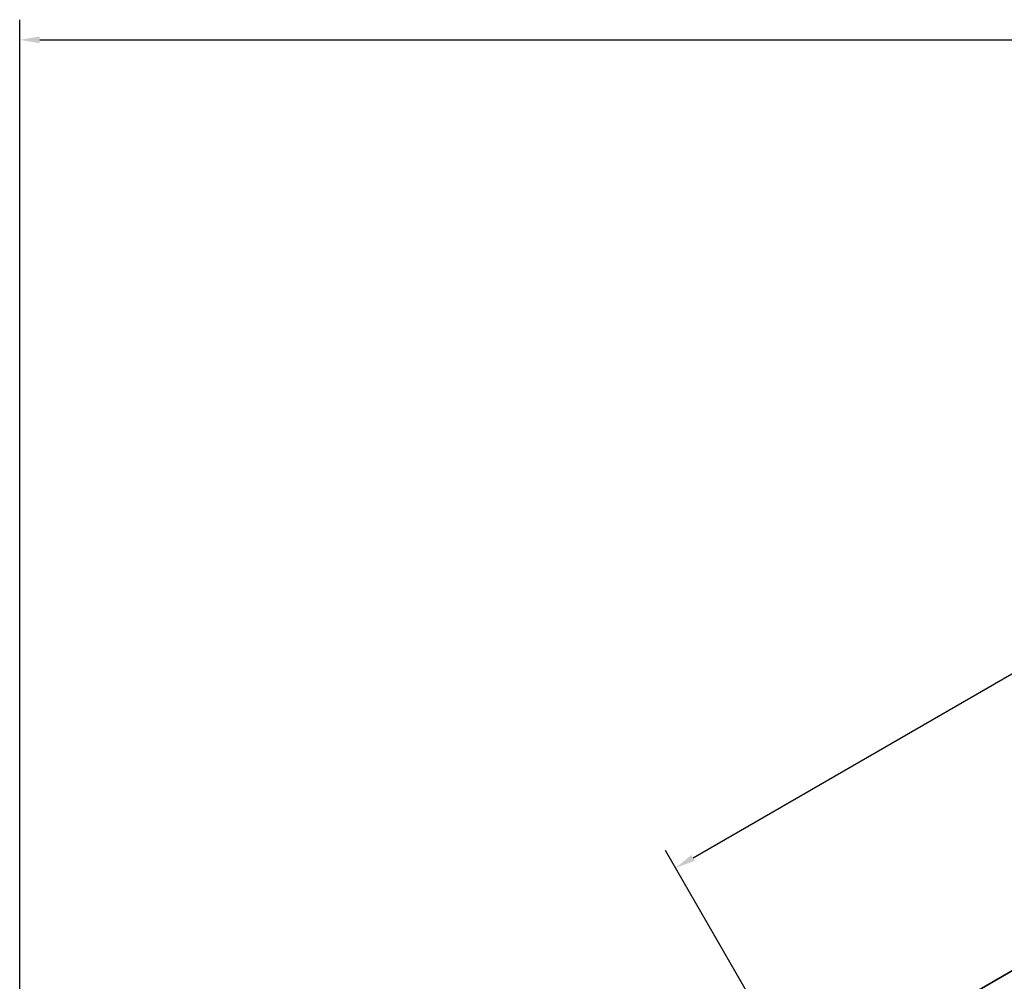
# Model space of a CAD drawing. Units: metres. Extents: x 12735 to 25554, y 20954 to 41989.
# Tile 9 of 15: x 12747.33 to 12756.135, y 20988.738 to 20997.336. Entities that reach past the tile are written whole.
import ezdxf

# ---------------------------------------------------------------- set-up
doc = ezdxf.new("R2010")
doc.units = ezdxf.units.M
doc.layers.get('Defpoints').update_dxf_attribs({"lineweight": 13})
doc.layers.add('A-ANNO-DIMS', color=2, linetype='Continuous', lineweight=18)
doc.layers.add('A-ELEV', color=7, linetype='Continuous', lineweight=35)
doc.styles.get("Standard").update_dxf_attribs({"font": 'arial.ttf'})
doc.dimstyles.get("Standard").update_dxf_attribs({"dimtxt": 0.18, "dimasz": 0.18, "dimexe": 0.18, "dimexo": 0.0625, "dimgap": 0.09, "dimtad": 0, "dimtih": 1, "dimtoh": 1, "dimdec": 4, "dimzin": 0, "dimdsep": 46, "dimtxsty": 'Standard', "dimcen": 0.09, "dimadec": 0, "dimazin": 0, "dimtfac": 1, "dimtdec": 4, "dimtofl": 0, "dimtmove": 0, "dimatfit": 3, "dimfxl": 1, "dimtolj": 1, "dimtzin": 0, "dimarcsym": 0})

# ---------------------------------------------------------------- blocks, each defined once
blk = doc.blocks.new('*D10')
at = {"layer": 'A-ANNO-DIMS', "color": 0, "lineweight": -2, "transparency": 16777216}
for p, q in [((12766.6445, 20994.8247), (12783.4841, 20994.8247)), ((12783.3041, 20994.6447), (12783.3041, 20975.781)), ((12783.3041, 20956.5534), (12783.3041, 20975.4171)), ((12755.8494, 20956.3734), (12783.4841, 20956.3734))]:
    blk.add_line(p, q, dxfattribs=at)
at = {"layer": 'A-ANNO-DIMS', "color": 0, "transparency": 16777216}
for points in [[(12783.2741, 20994.6447), (12783.3341, 20994.6447), (12783.3041, 20994.8247)], [(12783.2741, 20956.5534), (12783.3341, 20956.5534), (12783.3041, 20956.3734)]]:
    blk.add_solid(points, dxfattribs=at)
at = {"layer": 'Defpoints', "color": 0, "transparency": 16777216}
for p in [(12766.582, 20994.8247), (12783.3041, 20994.8247), (12755.7869, 20956.3734)]:
    blk.add_point(p, dxfattribs=at)
at = {"layer": 'A-ANNO-DIMS', "color": 0, "transparency": 16777216, "insert": (12783.3041, 20975.599), "char_height": 0.18, "attachment_point": 5}
blk.add_mtext('\\A1;38.45', dxfattribs=at)
blk = doc.blocks.new('*D17')
at = {"layer": 'A-ANNO-DIMS', "color": 0, "lineweight": -2, "transparency": 16777216}
for p, q in [((12766.6058, 20994.9106), (12765.397, 20997.0042)), ((12765.3311, 20996.7583), (12759.6564, 20993.482)), ((12753.3513, 20989.8417), (12759.026, 20993.118)), ((12754.3142, 20987.814), (12753.1054, 20989.9076))]:
    blk.add_line(p, q, dxfattribs=at)
at = {"layer": 'A-ANNO-DIMS', "color": 0, "transparency": 16777216}
for points in [[(12765.3161, 20996.7843), (12765.3461, 20996.7323), (12765.487, 20996.8483)], [(12753.3363, 20989.8677), (12753.3663, 20989.8157), (12753.1954, 20989.7517)]]:
    blk.add_solid(points, dxfattribs=at)
at = {"layer": 'Defpoints', "color": 0, "transparency": 16777216}
for p in [(12765.487, 20996.8483), (12766.637, 20994.8564), (12754.3454, 20987.7599)]:
    blk.add_point(p, dxfattribs=at)
at = {"layer": 'A-ANNO-DIMS', "color": 0, "transparency": 16777216, "insert": (12759.3412, 20993.3), "char_height": 0.18, "attachment_point": 5}
blk.add_mtext('\\A1;14.193', dxfattribs=at)
blk = doc.blocks.new('*D19')
at = {"layer": 'A-ANNO-DIMS', "color": 0, "lineweight": -2, "transparency": 16777216}
for p, q in [((12747.3297, 20976.0788), (12747.3297, 20997.3364)), ((12773.3057, 20974.7738), (12773.3057, 20997.3364)), ((12747.5097, 20997.1564), (12759.8526, 20997.1564)), ((12773.1257, 20997.1564), (12760.7828, 20997.1564))]:
    blk.add_line(p, q, dxfattribs=at)
at = {"layer": 'A-ANNO-DIMS', "color": 0, "transparency": 16777216}
for points in [[(12747.5097, 20997.1864), (12747.5097, 20997.1264), (12747.3297, 20997.1564)], [(12773.1257, 20997.1864), (12773.1257, 20997.1264), (12773.3057, 20997.1564)]]:
    blk.add_solid(points, dxfattribs=at)
at = {"layer": 'Defpoints', "color": 0, "transparency": 16777216}
for p in [(12773.3057, 20997.1564), (12747.3297, 20976.0163), (12773.3057, 20974.7113)]:
    blk.add_point(p, dxfattribs=at)
at = {"layer": 'A-ANNO-DIMS', "color": 0, "transparency": 16777216, "insert": (12760.3177, 20997.1564), "char_height": 0.18, "attachment_point": 5}
blk.add_mtext('\\A1;25.976', dxfattribs=at)

msp = doc.modelspace()

# ---------------------------------------------------------------- linework, layer by layer
at = {"layer": 'A-ELEV'}
msp.add_line((12754.3454, 20987.7599), (12766.637, 20994.8564), dxfattribs=at)

# ---------------------------------------------------------------- dimensions: what is measured, and where the dimension line sits
at = {"layer": 'A-ANNO-DIMS'}
dim = msp.add_linear_dim(base=(12773.3057, 20997.1564), p1=(12747.3297, 20976.0163), p2=(12773.3057, 20974.7113), dimstyle='Standard', override={"dimdec": 3, "dimlfac": 1, "dimrnd": 0, "dimzin": 0, "dimdsep": 46, "dimlunit": 2}, dxfattribs=at)
dim.commit()
dim.dimension.update_dxf_attribs({"geometry": '*D19', "text_midpoint": (12760.3177, 20997.1564)})
for base, p1, p2, angle, override, picture, middle in [((12765.487, 20996.8483), (12754.3454, 20987.7599), (12766.637, 20994.8564), 30, {"dimdec": 3, "dimlfac": 1, "dimrnd": 0, "dimzin": 0, "dimdsep": 46, "dimlunit": 2}, '*D17', (12759.3412, 20993.3)), ((12783.3041, 20994.8247), (12755.7869, 20956.3734), (12766.582, 20994.8247), 90, {"dimdec": 2, "dimlfac": 1, "dimrnd": 0, "dimzin": 0, "dimdsep": 46, "dimlunit": 2}, '*D10', (12783.3041, 20975.599))]:
    dim = msp.add_linear_dim(base=base, p1=p1, p2=p2, angle=angle, dimstyle='Standard', override=override, dxfattribs=at)
    dim.commit()
    dim.dimension.update_dxf_attribs({"geometry": picture, "text_midpoint": middle})

doc.saveas('drawing.dxf')
